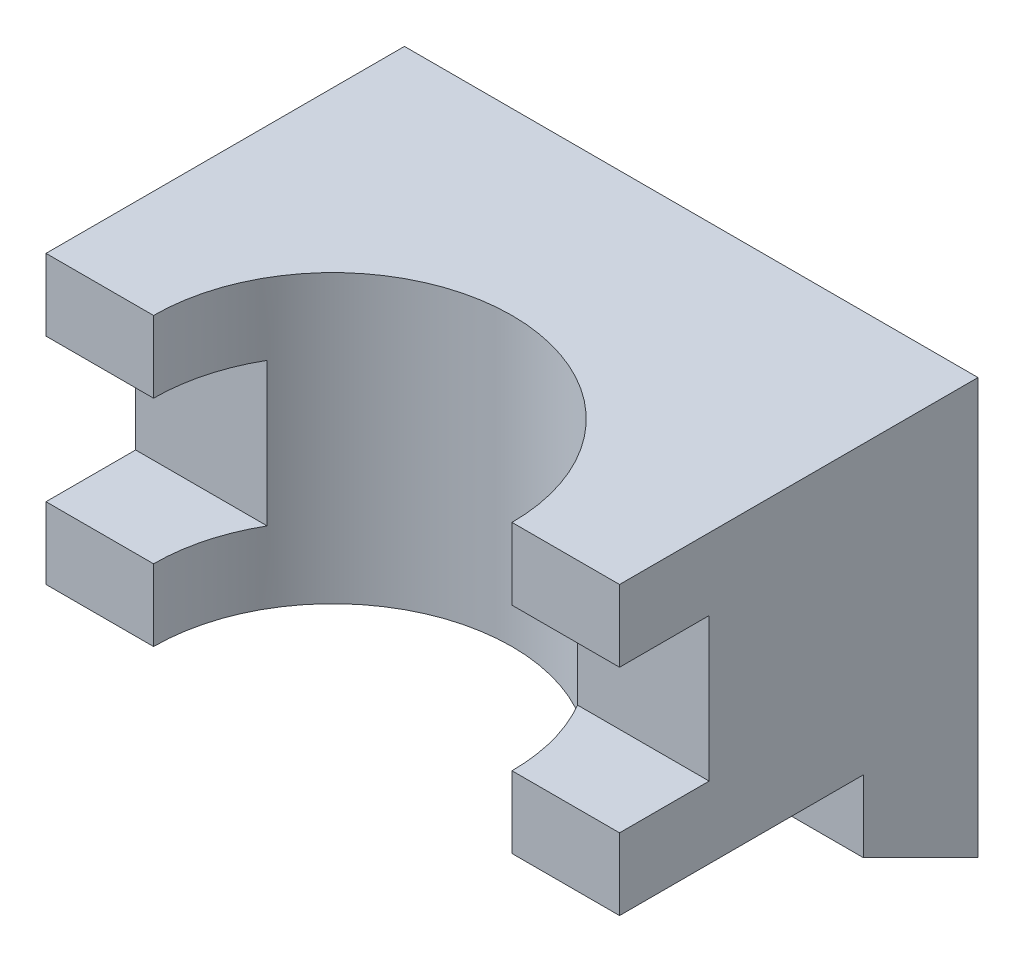
ISO-10303-21;
HEADER;
FILE_DESCRIPTION(('STEP AP214'),'2;1');
FILE_NAME('part.step','',(''),(''),'','','');
FILE_SCHEMA(('AUTOMOTIVE_DESIGN { 1 0 10303 214 1 1 1 1 }'));
ENDSEC;
DATA;
#1=APPLICATION_CONTEXT('core data for automotive mechanical design processes');
#2=APPLICATION_PROTOCOL_DEFINITION('international standard','automotive_design',2000,#1);
#3=PRODUCT_CONTEXT('',#1,'mechanical');
#4=PRODUCT('Part','Part','',(#3));
#5=PRODUCT_RELATED_PRODUCT_CATEGORY('part','',(#4));
#6=PRODUCT_DEFINITION_FORMATION('','',#4);
#7=PRODUCT_DEFINITION_CONTEXT('part definition',#1,'design');
#8=PRODUCT_DEFINITION('design','',#6,#7);
#9=PRODUCT_DEFINITION_SHAPE('','',#8);
#10=(LENGTH_UNIT() NAMED_UNIT(*) SI_UNIT(.MILLI.,.METRE.));
#11=(NAMED_UNIT(*) PLANE_ANGLE_UNIT() SI_UNIT($,.RADIAN.));
#12=(NAMED_UNIT(*) SI_UNIT($,.STERADIAN.) SOLID_ANGLE_UNIT());
#13=UNCERTAINTY_MEASURE_WITH_UNIT(LENGTH_MEASURE(1.E-05),#10,'distance_accuracy_value','');
#14=(GEOMETRIC_REPRESENTATION_CONTEXT(3) GLOBAL_UNCERTAINTY_ASSIGNED_CONTEXT((#13)) GLOBAL_UNIT_ASSIGNED_CONTEXT((#10,
#11,#12)) REPRESENTATION_CONTEXT('',''));
#15=CARTESIAN_POINT('',(0.,0.,0.));
#16=DIRECTION('',(0.,0.,1.));
#17=DIRECTION('',(1.,0.,0.));
#18=AXIS2_PLACEMENT_3D('',#15,#16,#17);
#19=CARTESIAN_POINT('',(80.,-30.,37.5));
#20=DIRECTION('',(0.,1.,0.));
#21=DIRECTION('',(0.,0.,1.));
#22=AXIS2_PLACEMENT_3D('',#19,#20,#21);
#23=PLANE('',#22);
#24=CARTESIAN_POINT('',(40.,-30.,50.));
#25=DIRECTION('',(0.,1.,0.));
#26=DIRECTION('',(0.,0.,1.));
#27=AXIS2_PLACEMENT_3D('',#24,#25,#26);
#28=CIRCLE('',#27,25.);
#29=CARTESIAN_POINT('',(18.349364905389,-30.,37.5));
#30=VERTEX_POINT('',#29);
#31=CARTESIAN_POINT('',(15.,-30.,50.));
#32=VERTEX_POINT('',#31);
#33=EDGE_CURVE('E232',#30,#32,#28,.T.);
#34=ORIENTED_EDGE('',*,*,#33,.F.);
#35=DIRECTION('',(-1.,0.,0.));
#36=VECTOR('',#35,1.);
#37=CARTESIAN_POINT('',(80.,-30.,37.5));
#38=LINE('',#37,#36);
#39=CARTESIAN_POINT('',(0.,-30.,37.5));
#40=VERTEX_POINT('',#39);
#41=EDGE_CURVE('E280',#30,#40,#38,.T.);
#42=ORIENTED_EDGE('',*,*,#41,.T.);
#43=DIRECTION('',(0.,0.,-1.));
#44=VECTOR('',#43,1.);
#45=CARTESIAN_POINT('',(0.,-30.,37.5));
#46=LINE('',#45,#44);
#47=CARTESIAN_POINT('',(0.,-30.,50.));
#48=VERTEX_POINT('',#47);
#49=EDGE_CURVE('E270',#48,#40,#46,.T.);
#50=ORIENTED_EDGE('',*,*,#49,.F.);
#51=DIRECTION('',(-1.,0.,0.));
#52=VECTOR('',#51,1.);
#53=CARTESIAN_POINT('',(80.,-30.,50.));
#54=LINE('',#53,#52);
#55=EDGE_CURVE('E283',#32,#48,#54,.T.);
#56=ORIENTED_EDGE('',*,*,#55,.F.);
#57=EDGE_LOOP('',(#34,#42,#50,#56));
#58=FACE_BOUND('',#57,.T.);
#59=ADVANCED_FACE('F44',(#58),#23,.T.);
#60=CARTESIAN_POINT('',(80.,-30.,50.));
#61=DIRECTION('',(0.,0.,1.));
#62=DIRECTION('',(1.,0.,0.));
#63=AXIS2_PLACEMENT_3D('',#60,#61,#62);
#64=PLANE('',#63);
#65=DIRECTION('',(0.,1.,0.));
#66=VECTOR('',#65,1.);
#67=CARTESIAN_POINT('',(15.,-40.,50.));
#68=LINE('',#67,#66);
#69=CARTESIAN_POINT('',(15.,-40.,50.));
#70=VERTEX_POINT('',#69);
#71=EDGE_CURVE('E240',#70,#32,#68,.T.);
#72=ORIENTED_EDGE('',*,*,#71,.T.);
#73=ORIENTED_EDGE('',*,*,#55,.T.);
#74=DIRECTION('',(0.,1.,0.));
#75=VECTOR('',#74,1.);
#76=CARTESIAN_POINT('',(0.,-30.,50.));
#77=LINE('',#76,#75);
#78=CARTESIAN_POINT('',(0.,-40.,50.));
#79=VERTEX_POINT('',#78);
#80=EDGE_CURVE('E264',#79,#48,#77,.T.);
#81=ORIENTED_EDGE('',*,*,#80,.F.);
#82=DIRECTION('',(-1.,0.,0.));
#83=VECTOR('',#82,1.);
#84=CARTESIAN_POINT('',(80.,-40.,50.));
#85=LINE('',#84,#83);
#86=EDGE_CURVE('E282',#70,#79,#85,.T.);
#87=ORIENTED_EDGE('',*,*,#86,.F.);
#88=EDGE_LOOP('',(#72,#73,#81,#87));
#89=FACE_BOUND('',#88,.T.);
#90=ADVANCED_FACE('F378',(#89),#64,.T.);
#91=CARTESIAN_POINT('',(80.,-10.,37.5));
#92=DIRECTION('',(0.,0.,1.));
#93=DIRECTION('',(1.,0.,0.));
#94=AXIS2_PLACEMENT_3D('',#91,#92,#93);
#95=PLANE('',#94);
#96=DIRECTION('',(0.,1.,0.));
#97=VECTOR('',#96,1.);
#98=CARTESIAN_POINT('',(61.650635094611,-40.,37.5));
#99=LINE('',#98,#97);
#100=CARTESIAN_POINT('',(61.650635094611,-30.,37.5));
#101=VERTEX_POINT('',#100);
#102=CARTESIAN_POINT('',(61.650635094611,-10.,37.5));
#103=VERTEX_POINT('',#102);
#104=EDGE_CURVE('E246',#101,#103,#99,.T.);
#105=ORIENTED_EDGE('',*,*,#104,.F.);
#106=CARTESIAN_POINT('',(80.,-30.,37.5));
#107=VERTEX_POINT('',#106);
#108=EDGE_CURVE('E274',#107,#101,#38,.T.);
#109=ORIENTED_EDGE('',*,*,#108,.F.);
#110=DIRECTION('',(0.,1.,0.));
#111=VECTOR('',#110,1.);
#112=CARTESIAN_POINT('',(80.,-10.,37.5));
#113=LINE('',#112,#111);
#114=CARTESIAN_POINT('',(80.,-10.,37.5));
#115=VERTEX_POINT('',#114);
#116=EDGE_CURVE('E256',#107,#115,#113,.T.);
#117=ORIENTED_EDGE('',*,*,#116,.T.);
#118=DIRECTION('',(-1.,0.,0.));
#119=VECTOR('',#118,1.);
#120=CARTESIAN_POINT('',(80.,-10.,37.5));
#121=LINE('',#120,#119);
#122=EDGE_CURVE('E268',#115,#103,#121,.T.);
#123=ORIENTED_EDGE('',*,*,#122,.T.);
#124=EDGE_LOOP('',(#105,#109,#117,#123));
#125=FACE_BOUND('',#124,.T.);
#126=ADVANCED_FACE('F415',(#125),#95,.T.);
#127=CARTESIAN_POINT('',(40.,-10.,50.));
#128=DIRECTION('',(0.,1.,0.));
#129=DIRECTION('',(0.,0.,1.));
#130=AXIS2_PLACEMENT_3D('',#127,#128,#129);
#131=PLANE('',#130);
#132=DIRECTION('',(0.,0.,1.));
#133=VECTOR('',#132,1.);
#134=CARTESIAN_POINT('',(0.,-10.,16.));
#135=LINE('',#134,#133);
#136=CARTESIAN_POINT('',(0.,-10.,37.5));
#137=VERTEX_POINT('',#136);
#138=CARTESIAN_POINT('',(0.,-10.,50.));
#139=VERTEX_POINT('',#138);
#140=EDGE_CURVE('E305',#137,#139,#135,.T.);
#141=ORIENTED_EDGE('',*,*,#140,.F.);
#142=DIRECTION('',(1.,0.,0.));
#143=VECTOR('',#142,1.);
#144=CARTESIAN_POINT('',(40.,-10.,37.5));
#145=LINE('',#144,#143);
#146=CARTESIAN_POINT('',(18.349364905389,-10.,37.5));
#147=VERTEX_POINT('',#146);
#148=EDGE_CURVE('E345',#137,#147,#145,.T.);
#149=ORIENTED_EDGE('',*,*,#148,.T.);
#150=CARTESIAN_POINT('',(40.,-10.,50.));
#151=DIRECTION('',(0.,-1.,0.));
#152=DIRECTION('',(0.,0.,1.));
#153=AXIS2_PLACEMENT_3D('',#150,#151,#152);
#154=CIRCLE('',#153,25.);
#155=CARTESIAN_POINT('',(15.,-10.,50.));
#156=VERTEX_POINT('',#155);
#157=EDGE_CURVE('E291',#156,#147,#154,.T.);
#158=ORIENTED_EDGE('',*,*,#157,.F.);
#159=DIRECTION('',(1.,0.,0.));
#160=VECTOR('',#159,1.);
#161=CARTESIAN_POINT('',(0.,-10.,50.));
#162=LINE('',#161,#160);
#163=EDGE_CURVE('E289',#139,#156,#162,.T.);
#164=ORIENTED_EDGE('',*,*,#163,.F.);
#165=EDGE_LOOP('',(#141,#149,#158,#164));
#166=FACE_BOUND('',#165,.T.);
#167=ADVANCED_FACE('F393',(#166),#131,.F.);
#168=CARTESIAN_POINT('',(0.,0.,16.));
#169=DIRECTION('',(0.,-1.,0.));
#170=DIRECTION('',(0.,0.,-1.));
#171=AXIS2_PLACEMENT_3D('',#168,#169,#170);
#172=PLANE('',#171);
#173=DIRECTION('',(-1.,0.,0.));
#174=VECTOR('',#173,1.);
#175=CARTESIAN_POINT('',(0.,0.,0.));
#176=LINE('',#175,#174);
#177=CARTESIAN_POINT('',(80.,0.,0.));
#178=VERTEX_POINT('',#177);
#179=CARTESIAN_POINT('',(0.,0.,0.));
#180=VERTEX_POINT('',#179);
#181=EDGE_CURVE('E314',#178,#180,#176,.T.);
#182=ORIENTED_EDGE('',*,*,#181,.T.);
#183=DIRECTION('',(0.,0.,-1.));
#184=VECTOR('',#183,1.);
#185=CARTESIAN_POINT('',(0.,0.,16.));
#186=LINE('',#185,#184);
#187=CARTESIAN_POINT('',(0.,0.,50.));
#188=VERTEX_POINT('',#187);
#189=EDGE_CURVE('E339',#188,#180,#186,.T.);
#190=ORIENTED_EDGE('',*,*,#189,.F.);
#191=DIRECTION('',(1.,0.,0.));
#192=VECTOR('',#191,1.);
#193=CARTESIAN_POINT('',(0.,0.,50.));
#194=LINE('',#193,#192);
#195=CARTESIAN_POINT('',(15.,0.,50.));
#196=VERTEX_POINT('',#195);
#197=EDGE_CURVE('E271',#188,#196,#194,.T.);
#198=ORIENTED_EDGE('',*,*,#197,.T.);
#199=CARTESIAN_POINT('',(40.,0.,50.));
#200=DIRECTION('',(0.,-1.,0.));
#201=DIRECTION('',(0.,0.,1.));
#202=AXIS2_PLACEMENT_3D('',#199,#200,#201);
#203=CIRCLE('',#202,25.);
#204=CARTESIAN_POINT('',(65.,0.,50.));
#205=VERTEX_POINT('',#204);
#206=EDGE_CURVE('E310',#196,#205,#203,.T.);
#207=ORIENTED_EDGE('',*,*,#206,.T.);
#208=DIRECTION('',(1.,0.,0.));
#209=VECTOR('',#208,1.);
#210=CARTESIAN_POINT('',(65.,0.,50.));
#211=LINE('',#210,#209);
#212=CARTESIAN_POINT('',(80.,0.,50.));
#213=VERTEX_POINT('',#212);
#214=EDGE_CURVE('E292',#205,#213,#211,.T.);
#215=ORIENTED_EDGE('',*,*,#214,.T.);
#216=DIRECTION('',(0.,0.,-1.));
#217=VECTOR('',#216,1.);
#218=CARTESIAN_POINT('',(80.,0.,16.));
#219=LINE('',#218,#217);
#220=EDGE_CURVE('E326',#213,#178,#219,.T.);
#221=ORIENTED_EDGE('',*,*,#220,.T.);
#222=EDGE_LOOP('',(#182,#190,#198,#207,#215,#221));
#223=FACE_BOUND('',#222,.T.);
#224=ADVANCED_FACE('F50',(#223),#172,.F.);
#225=CARTESIAN_POINT('',(0.,0.,16.));
#226=DIRECTION('',(1.,0.,0.));
#227=DIRECTION('',(0.,0.,-1.));
#228=AXIS2_PLACEMENT_3D('',#225,#226,#227);
#229=PLANE('',#228);
#230=DIRECTION('',(0.,-1.,0.));
#231=VECTOR('',#230,1.);
#232=CARTESIAN_POINT('',(0.,0.,0.));
#233=LINE('',#232,#231);
#234=CARTESIAN_POINT('',(0.,-58.,0.));
#235=VERTEX_POINT('',#234);
#236=EDGE_CURVE('E332',#180,#235,#233,.T.);
#237=ORIENTED_EDGE('',*,*,#236,.T.);
#238=DIRECTION('',(0.,-0.447213595499958,-0.894427190999916));
#239=VECTOR('',#238,1.);
#240=CARTESIAN_POINT('',(0.,-50.,16.));
#241=LINE('',#240,#239);
#242=CARTESIAN_POINT('',(0.,-50.,16.));
#243=VERTEX_POINT('',#242);
#244=EDGE_CURVE('E222',#243,#235,#241,.T.);
#245=ORIENTED_EDGE('',*,*,#244,.F.);
#246=DIRECTION('',(0.,-1.,0.));
#247=VECTOR('',#246,1.);
#248=CARTESIAN_POINT('',(0.,0.,16.));
#249=LINE('',#248,#247);
#250=CARTESIAN_POINT('',(0.,-40.,16.));
#251=VERTEX_POINT('',#250);
#252=EDGE_CURVE('E325',#251,#243,#249,.T.);
#253=ORIENTED_EDGE('',*,*,#252,.F.);
#254=DIRECTION('',(0.,0.,1.));
#255=VECTOR('',#254,1.);
#256=CARTESIAN_POINT('',(0.,-40.,50.));
#257=LINE('',#256,#255);
#258=EDGE_CURVE('E247',#251,#79,#257,.T.);
#259=ORIENTED_EDGE('',*,*,#258,.T.);
#260=ORIENTED_EDGE('',*,*,#80,.T.);
#261=ORIENTED_EDGE('',*,*,#49,.T.);
#262=DIRECTION('',(0.,1.,0.));
#263=VECTOR('',#262,1.);
#264=CARTESIAN_POINT('',(0.,-10.,37.5));
#265=LINE('',#264,#263);
#266=EDGE_CURVE('E66',#40,#137,#265,.T.);
#267=ORIENTED_EDGE('',*,*,#266,.T.);
#268=ORIENTED_EDGE('',*,*,#140,.T.);
#269=DIRECTION('',(0.,1.,0.));
#270=VECTOR('',#269,1.);
#271=CARTESIAN_POINT('',(0.,-10.,50.));
#272=LINE('',#271,#270);
#273=EDGE_CURVE('E315',#139,#188,#272,.T.);
#274=ORIENTED_EDGE('',*,*,#273,.T.);
#275=ORIENTED_EDGE('',*,*,#189,.T.);
#276=EDGE_LOOP('',(#237,#245,#253,#259,#260,#261,#267,#268,#274,#275));
#277=FACE_BOUND('',#276,.T.);
#278=ADVANCED_FACE('F359',(#277),#229,.F.);
#279=CARTESIAN_POINT('',(80.,0.,16.));
#280=DIRECTION('',(-1.,0.,0.));
#281=DIRECTION('',(0.,0.,1.));
#282=AXIS2_PLACEMENT_3D('',#279,#280,#281);
#283=PLANE('',#282);
#284=DIRECTION('',(0.,1.,0.));
#285=VECTOR('',#284,1.);
#286=CARTESIAN_POINT('',(80.,0.,16.));
#287=LINE('',#286,#285);
#288=CARTESIAN_POINT('',(80.,-50.,16.));
#289=VERTEX_POINT('',#288);
#290=CARTESIAN_POINT('',(80.,-40.,16.));
#291=VERTEX_POINT('',#290);
#292=EDGE_CURVE('E323',#289,#291,#287,.T.);
#293=ORIENTED_EDGE('',*,*,#292,.F.);
#294=DIRECTION('',(0.,-0.447213595499958,-0.894427190999916));
#295=VECTOR('',#294,1.);
#296=CARTESIAN_POINT('',(80.,-50.,16.));
#297=LINE('',#296,#295);
#298=CARTESIAN_POINT('',(80.,-58.,0.));
#299=VERTEX_POINT('',#298);
#300=EDGE_CURVE('E228',#289,#299,#297,.T.);
#301=ORIENTED_EDGE('',*,*,#300,.T.);
#302=DIRECTION('',(0.,1.,0.));
#303=VECTOR('',#302,1.);
#304=CARTESIAN_POINT('',(80.,0.,0.));
#305=LINE('',#304,#303);
#306=EDGE_CURVE('E328',#299,#178,#305,.T.);
#307=ORIENTED_EDGE('',*,*,#306,.T.);
#308=ORIENTED_EDGE('',*,*,#220,.F.);
#309=DIRECTION('',(0.,1.,0.));
#310=VECTOR('',#309,1.);
#311=CARTESIAN_POINT('',(80.,-10.,50.));
#312=LINE('',#311,#310);
#313=CARTESIAN_POINT('',(80.,-10.,50.));
#314=VERTEX_POINT('',#313);
#315=EDGE_CURVE('E317',#314,#213,#312,.T.);
#316=ORIENTED_EDGE('',*,*,#315,.F.);
#317=DIRECTION('',(0.,0.,-1.));
#318=VECTOR('',#317,1.);
#319=CARTESIAN_POINT('',(80.,-10.,50.));
#320=LINE('',#319,#318);
#321=EDGE_CURVE('E299',#314,#115,#320,.T.);
#322=ORIENTED_EDGE('',*,*,#321,.T.);
#323=ORIENTED_EDGE('',*,*,#116,.F.);
#324=DIRECTION('',(0.,0.,-1.));
#325=VECTOR('',#324,1.);
#326=CARTESIAN_POINT('',(80.,-30.,37.5));
#327=LINE('',#326,#325);
#328=CARTESIAN_POINT('',(80.,-30.,50.));
#329=VERTEX_POINT('',#328);
#330=EDGE_CURVE('E257',#329,#107,#327,.T.);
#331=ORIENTED_EDGE('',*,*,#330,.F.);
#332=DIRECTION('',(0.,1.,0.));
#333=VECTOR('',#332,1.);
#334=CARTESIAN_POINT('',(80.,-30.,50.));
#335=LINE('',#334,#333);
#336=CARTESIAN_POINT('',(80.,-40.,50.));
#337=VERTEX_POINT('',#336);
#338=EDGE_CURVE('E254',#337,#329,#335,.T.);
#339=ORIENTED_EDGE('',*,*,#338,.F.);
#340=DIRECTION('',(0.,0.,1.));
#341=VECTOR('',#340,1.);
#342=CARTESIAN_POINT('',(80.,-40.,50.));
#343=LINE('',#342,#341);
#344=EDGE_CURVE('E249',#291,#337,#343,.T.);
#345=ORIENTED_EDGE('',*,*,#344,.F.);
#346=EDGE_LOOP('',(#293,#301,#307,#308,#316,#322,#323,#331,#339,#345));
#347=FACE_BOUND('',#346,.T.);
#348=ADVANCED_FACE('F367',(#347),#283,.F.);
#349=CARTESIAN_POINT('',(0.,0.,16.));
#350=DIRECTION('',(0.,0.,-1.));
#351=DIRECTION('',(-1.,0.,0.));
#352=AXIS2_PLACEMENT_3D('',#349,#350,#351);
#353=PLANE('',#352);
#354=DIRECTION('',(-1.,0.,0.));
#355=VECTOR('',#354,1.);
#356=CARTESIAN_POINT('',(80.,-50.,16.));
#357=LINE('',#356,#355);
#358=CARTESIAN_POINT('',(20.,-50.,16.));
#359=VERTEX_POINT('',#358);
#360=EDGE_CURVE('E230',#359,#243,#357,.T.);
#361=ORIENTED_EDGE('',*,*,#360,.F.);
#362=DIRECTION('',(0.,-1.,0.));
#363=VECTOR('',#362,1.);
#364=CARTESIAN_POINT('',(20.,-45.,16.));
#365=LINE('',#364,#363);
#366=CARTESIAN_POINT('',(20.,-45.,16.));
#367=VERTEX_POINT('',#366);
#368=EDGE_CURVE('E200',#367,#359,#365,.T.);
#369=ORIENTED_EDGE('',*,*,#368,.F.);
#370=DIRECTION('',(-1.,0.,0.));
#371=VECTOR('',#370,1.);
#372=CARTESIAN_POINT('',(60.,-45.,16.));
#373=LINE('',#372,#371);
#374=CARTESIAN_POINT('',(60.,-45.,16.));
#375=VERTEX_POINT('',#374);
#376=EDGE_CURVE('E220',#375,#367,#373,.T.);
#377=ORIENTED_EDGE('',*,*,#376,.F.);
#378=DIRECTION('',(0.,1.,0.));
#379=VECTOR('',#378,1.);
#380=CARTESIAN_POINT('',(60.,-50.,16.));
#381=LINE('',#380,#379);
#382=CARTESIAN_POINT('',(60.,-50.,16.));
#383=VERTEX_POINT('',#382);
#384=EDGE_CURVE('E204',#383,#375,#381,.T.);
#385=ORIENTED_EDGE('',*,*,#384,.F.);
#386=EDGE_CURVE('E233',#289,#383,#357,.T.);
#387=ORIENTED_EDGE('',*,*,#386,.F.);
#388=ORIENTED_EDGE('',*,*,#292,.T.);
#389=DIRECTION('',(-1.,0.,0.));
#390=VECTOR('',#389,1.);
#391=CARTESIAN_POINT('',(80.,-40.,16.));
#392=LINE('',#391,#390);
#393=EDGE_CURVE('E263',#291,#251,#392,.T.);
#394=ORIENTED_EDGE('',*,*,#393,.T.);
#395=ORIENTED_EDGE('',*,*,#252,.T.);
#396=EDGE_LOOP('',(#361,#369,#377,#385,#387,#388,#394,#395));
#397=FACE_BOUND('',#396,.T.);
#398=ADVANCED_FACE('F357',(#397),#353,.F.);
#399=CARTESIAN_POINT('',(0.,0.,0.));
#400=DIRECTION('',(0.,0.,-1.));
#401=DIRECTION('',(-1.,0.,0.));
#402=AXIS2_PLACEMENT_3D('',#399,#400,#401);
#403=PLANE('',#402);
#404=ORIENTED_EDGE('',*,*,#181,.F.);
#405=ORIENTED_EDGE('',*,*,#306,.F.);
#406=DIRECTION('',(1.,0.,0.));
#407=VECTOR('',#406,1.);
#408=CARTESIAN_POINT('',(80.,-58.,0.));
#409=LINE('',#408,#407);
#410=EDGE_CURVE('E331',#235,#299,#409,.T.);
#411=ORIENTED_EDGE('',*,*,#410,.F.);
#412=ORIENTED_EDGE('',*,*,#236,.F.);
#413=EDGE_LOOP('',(#404,#405,#411,#412));
#414=FACE_BOUND('',#413,.T.);
#415=ADVANCED_FACE('F362',(#414),#403,.T.);
#416=CARTESIAN_POINT('',(0.,-10.,50.));
#417=DIRECTION('',(0.,0.,1.));
#418=DIRECTION('',(1.,0.,0.));
#419=AXIS2_PLACEMENT_3D('',#416,#417,#418);
#420=PLANE('',#419);
#421=ORIENTED_EDGE('',*,*,#197,.F.);
#422=ORIENTED_EDGE('',*,*,#273,.F.);
#423=ORIENTED_EDGE('',*,*,#163,.T.);
#424=DIRECTION('',(0.,1.,0.));
#425=VECTOR('',#424,1.);
#426=CARTESIAN_POINT('',(15.,-10.,50.));
#427=LINE('',#426,#425);
#428=EDGE_CURVE('E302',#156,#196,#427,.T.);
#429=ORIENTED_EDGE('',*,*,#428,.T.);
#430=EDGE_LOOP('',(#421,#422,#423,#429));
#431=FACE_BOUND('',#430,.T.);
#432=ADVANCED_FACE('F392',(#431),#420,.T.);
#433=CARTESIAN_POINT('',(65.,-10.,50.));
#434=DIRECTION('',(0.,0.,1.));
#435=DIRECTION('',(1.,0.,0.));
#436=AXIS2_PLACEMENT_3D('',#433,#434,#435);
#437=PLANE('',#436);
#438=ORIENTED_EDGE('',*,*,#214,.F.);
#439=DIRECTION('',(0.,1.,0.));
#440=VECTOR('',#439,1.);
#441=CARTESIAN_POINT('',(65.,-10.,50.));
#442=LINE('',#441,#440);
#443=CARTESIAN_POINT('',(65.,-10.,50.));
#444=VERTEX_POINT('',#443);
#445=EDGE_CURVE('E316',#444,#205,#442,.T.);
#446=ORIENTED_EDGE('',*,*,#445,.F.);
#447=DIRECTION('',(1.,0.,0.));
#448=VECTOR('',#447,1.);
#449=CARTESIAN_POINT('',(65.,-10.,50.));
#450=LINE('',#449,#448);
#451=EDGE_CURVE('E298',#444,#314,#450,.T.);
#452=ORIENTED_EDGE('',*,*,#451,.T.);
#453=ORIENTED_EDGE('',*,*,#315,.T.);
#454=EDGE_LOOP('',(#438,#446,#452,#453));
#455=FACE_BOUND('',#454,.T.);
#456=ADVANCED_FACE('F402',(#455),#437,.T.);
#457=CARTESIAN_POINT('',(40.,-10.,50.));
#458=DIRECTION('',(0.,1.,0.));
#459=DIRECTION('',(0.,0.,1.));
#460=AXIS2_PLACEMENT_3D('',#457,#458,#459);
#461=CYLINDRICAL_SURFACE('',#460,25.);
#462=ORIENTED_EDGE('',*,*,#206,.F.);
#463=ORIENTED_EDGE('',*,*,#428,.F.);
#464=ORIENTED_EDGE('',*,*,#157,.T.);
#465=DIRECTION('',(0.,1.,0.));
#466=VECTOR('',#465,1.);
#467=CARTESIAN_POINT('',(18.349364905389,-40.,37.5));
#468=LINE('',#467,#466);
#469=EDGE_CURVE('E244',#30,#147,#468,.T.);
#470=ORIENTED_EDGE('',*,*,#469,.F.);
#471=ORIENTED_EDGE('',*,*,#33,.T.);
#472=ORIENTED_EDGE('',*,*,#71,.F.);
#473=CARTESIAN_POINT('',(40.,-40.,50.));
#474=DIRECTION('',(0.,1.,0.));
#475=DIRECTION('',(0.,0.,1.));
#476=AXIS2_PLACEMENT_3D('',#473,#474,#475);
#477=CIRCLE('',#476,25.);
#478=CARTESIAN_POINT('',(65.,-40.,50.));
#479=VERTEX_POINT('',#478);
#480=EDGE_CURVE('E241',#479,#70,#477,.T.);
#481=ORIENTED_EDGE('',*,*,#480,.F.);
#482=DIRECTION('',(0.,1.,0.));
#483=VECTOR('',#482,1.);
#484=CARTESIAN_POINT('',(65.,-40.,50.));
#485=LINE('',#484,#483);
#486=CARTESIAN_POINT('',(65.,-30.,50.));
#487=VERTEX_POINT('',#486);
#488=EDGE_CURVE('E238',#479,#487,#485,.T.);
#489=ORIENTED_EDGE('',*,*,#488,.T.);
#490=CARTESIAN_POINT('',(40.,-30.,50.));
#491=DIRECTION('',(0.,1.,0.));
#492=DIRECTION('',(0.,0.,1.));
#493=AXIS2_PLACEMENT_3D('',#490,#491,#492);
#494=CIRCLE('',#493,25.);
#495=EDGE_CURVE('E234',#487,#101,#494,.T.);
#496=ORIENTED_EDGE('',*,*,#495,.T.);
#497=ORIENTED_EDGE('',*,*,#104,.T.);
#498=EDGE_CURVE('E293',#103,#444,#154,.T.);
#499=ORIENTED_EDGE('',*,*,#498,.T.);
#500=ORIENTED_EDGE('',*,*,#445,.T.);
#501=EDGE_LOOP('',(#462,#463,#464,#470,#471,#472,#481,#489,#496,#497,#499,#500));
#502=FACE_BOUND('',#501,.T.);
#503=ADVANCED_FACE('F418',(#502),#461,.F.);
#504=ORIENTED_EDGE('',*,*,#498,.F.);
#505=ORIENTED_EDGE('',*,*,#122,.F.);
#506=ORIENTED_EDGE('',*,*,#321,.F.);
#507=ORIENTED_EDGE('',*,*,#451,.F.);
#508=EDGE_LOOP('',(#504,#505,#506,#507));
#509=FACE_BOUND('',#508,.T.);
#510=ADVANCED_FACE('F407',(#509),#131,.F.);
#511=ORIENTED_EDGE('',*,*,#469,.T.);
#512=ORIENTED_EDGE('',*,*,#148,.F.);
#513=ORIENTED_EDGE('',*,*,#266,.F.);
#514=ORIENTED_EDGE('',*,*,#41,.F.);
#515=EDGE_LOOP('',(#511,#512,#513,#514));
#516=FACE_BOUND('',#515,.T.);
#517=ADVANCED_FACE('F387',(#516),#95,.T.);
#518=ORIENTED_EDGE('',*,*,#495,.F.);
#519=EDGE_CURVE('E279',#329,#487,#54,.T.);
#520=ORIENTED_EDGE('',*,*,#519,.F.);
#521=ORIENTED_EDGE('',*,*,#330,.T.);
#522=ORIENTED_EDGE('',*,*,#108,.T.);
#523=EDGE_LOOP('',(#518,#520,#521,#522));
#524=FACE_BOUND('',#523,.T.);
#525=ADVANCED_FACE('F412',(#524),#23,.T.);
#526=ORIENTED_EDGE('',*,*,#488,.F.);
#527=EDGE_CURVE('E285',#337,#479,#85,.T.);
#528=ORIENTED_EDGE('',*,*,#527,.F.);
#529=ORIENTED_EDGE('',*,*,#338,.T.);
#530=ORIENTED_EDGE('',*,*,#519,.T.);
#531=EDGE_LOOP('',(#526,#528,#529,#530));
#532=FACE_BOUND('',#531,.T.);
#533=ADVANCED_FACE('F419',(#532),#64,.T.);
#534=CARTESIAN_POINT('',(80.,-40.,50.));
#535=DIRECTION('',(0.,-1.,0.));
#536=DIRECTION('',(0.,0.,-1.));
#537=AXIS2_PLACEMENT_3D('',#534,#535,#536);
#538=PLANE('',#537);
#539=ORIENTED_EDGE('',*,*,#480,.T.);
#540=ORIENTED_EDGE('',*,*,#86,.T.);
#541=ORIENTED_EDGE('',*,*,#258,.F.);
#542=ORIENTED_EDGE('',*,*,#393,.F.);
#543=ORIENTED_EDGE('',*,*,#344,.T.);
#544=ORIENTED_EDGE('',*,*,#527,.T.);
#545=EDGE_LOOP('',(#539,#540,#541,#542,#543,#544));
#546=FACE_BOUND('',#545,.T.);
#547=ADVANCED_FACE('F372',(#546),#538,.T.);
#548=CARTESIAN_POINT('',(80.,-50.,16.));
#549=DIRECTION('',(0.,0.894427190999916,-0.447213595499958));
#550=DIRECTION('',(0.,0.447213595499958,0.894427190999916));
#551=AXIS2_PLACEMENT_3D('',#548,#549,#550);
#552=PLANE('',#551);
#553=DIRECTION('',(-1.,0.,0.));
#554=VECTOR('',#553,1.);
#555=CARTESIAN_POINT('',(80.,-55.,5.99999999999998));
#556=LINE('',#555,#554);
#557=CARTESIAN_POINT('',(60.,-55.,5.99999999999998));
#558=VERTEX_POINT('',#557);
#559=CARTESIAN_POINT('',(20.,-55.,5.99999999999996));
#560=VERTEX_POINT('',#559);
#561=EDGE_CURVE('E52',#558,#560,#556,.T.);
#562=ORIENTED_EDGE('',*,*,#561,.T.);
#563=DIRECTION('',(0.,0.447213595499958,0.894427190999916));
#564=VECTOR('',#563,1.);
#565=CARTESIAN_POINT('',(20.,-50.,16.));
#566=LINE('',#565,#564);
#567=EDGE_CURVE('E11',#560,#359,#566,.T.);
#568=ORIENTED_EDGE('',*,*,#567,.T.);
#569=ORIENTED_EDGE('',*,*,#360,.T.);
#570=ORIENTED_EDGE('',*,*,#244,.T.);
#571=ORIENTED_EDGE('',*,*,#410,.T.);
#572=ORIENTED_EDGE('',*,*,#300,.F.);
#573=ORIENTED_EDGE('',*,*,#386,.T.);
#574=DIRECTION('',(0.,-0.447213595499958,-0.894427190999916));
#575=VECTOR('',#574,1.);
#576=CARTESIAN_POINT('',(60.,-50.,16.));
#577=LINE('',#576,#575);
#578=EDGE_CURVE('E343',#383,#558,#577,.T.);
#579=ORIENTED_EDGE('',*,*,#578,.T.);
#580=EDGE_LOOP('',(#562,#568,#569,#570,#571,#572,#573,#579));
#581=FACE_BOUND('',#580,.T.);
#582=ADVANCED_FACE('F349',(#581),#552,.F.);
#583=CARTESIAN_POINT('',(20.,-55.,5.));
#584=DIRECTION('',(0.,-1.,0.));
#585=DIRECTION('',(0.,0.,-1.));
#586=AXIS2_PLACEMENT_3D('',#583,#584,#585);
#587=PLANE('',#586);
#588=DIRECTION('',(0.,0.,1.));
#589=VECTOR('',#588,1.);
#590=CARTESIAN_POINT('',(60.,-55.,5.));
#591=LINE('',#590,#589);
#592=CARTESIAN_POINT('',(60.,-55.,5.));
#593=VERTEX_POINT('',#592);
#594=EDGE_CURVE('E58',#593,#558,#591,.T.);
#595=ORIENTED_EDGE('',*,*,#594,.F.);
#596=DIRECTION('',(1.,0.,0.));
#597=VECTOR('',#596,1.);
#598=CARTESIAN_POINT('',(20.,-55.,5.));
#599=LINE('',#598,#597);
#600=CARTESIAN_POINT('',(20.,-55.,5.));
#601=VERTEX_POINT('',#600);
#602=EDGE_CURVE('E198',#601,#593,#599,.T.);
#603=ORIENTED_EDGE('',*,*,#602,.F.);
#604=DIRECTION('',(0.,0.,1.));
#605=VECTOR('',#604,1.);
#606=CARTESIAN_POINT('',(20.,-55.,5.));
#607=LINE('',#606,#605);
#608=EDGE_CURVE('E225',#601,#560,#607,.T.);
#609=ORIENTED_EDGE('',*,*,#608,.T.);
#610=ORIENTED_EDGE('',*,*,#561,.F.);
#611=EDGE_LOOP('',(#595,#603,#609,#610));
#612=FACE_BOUND('',#611,.T.);
#613=ADVANCED_FACE('F355',(#612),#587,.F.);
#614=CARTESIAN_POINT('',(20.,-45.,5.));
#615=DIRECTION('',(-1.,0.,0.));
#616=DIRECTION('',(0.,0.,1.));
#617=AXIS2_PLACEMENT_3D('',#614,#615,#616);
#618=PLANE('',#617);
#619=ORIENTED_EDGE('',*,*,#608,.F.);
#620=DIRECTION('',(0.,-1.,0.));
#621=VECTOR('',#620,1.);
#622=CARTESIAN_POINT('',(20.,-45.,5.));
#623=LINE('',#622,#621);
#624=CARTESIAN_POINT('',(20.,-45.,5.));
#625=VERTEX_POINT('',#624);
#626=EDGE_CURVE('E212',#625,#601,#623,.T.);
#627=ORIENTED_EDGE('',*,*,#626,.F.);
#628=DIRECTION('',(0.,0.,1.));
#629=VECTOR('',#628,1.);
#630=CARTESIAN_POINT('',(20.,-45.,5.));
#631=LINE('',#630,#629);
#632=EDGE_CURVE('E210',#625,#367,#631,.T.);
#633=ORIENTED_EDGE('',*,*,#632,.T.);
#634=ORIENTED_EDGE('',*,*,#368,.T.);
#635=ORIENTED_EDGE('',*,*,#567,.F.);
#636=EDGE_LOOP('',(#619,#627,#633,#634,#635));
#637=FACE_BOUND('',#636,.T.);
#638=ADVANCED_FACE('F351',(#637),#618,.F.);
#639=CARTESIAN_POINT('',(60.,-50.,5.));
#640=DIRECTION('',(1.,0.,0.));
#641=DIRECTION('',(0.,0.,-1.));
#642=AXIS2_PLACEMENT_3D('',#639,#640,#641);
#643=PLANE('',#642);
#644=ORIENTED_EDGE('',*,*,#384,.T.);
#645=DIRECTION('',(0.,0.,1.));
#646=VECTOR('',#645,1.);
#647=CARTESIAN_POINT('',(60.,-45.,5.));
#648=LINE('',#647,#646);
#649=CARTESIAN_POINT('',(60.,-45.,5.));
#650=VERTEX_POINT('',#649);
#651=EDGE_CURVE('E197',#650,#375,#648,.T.);
#652=ORIENTED_EDGE('',*,*,#651,.F.);
#653=DIRECTION('',(0.,1.,0.));
#654=VECTOR('',#653,1.);
#655=CARTESIAN_POINT('',(60.,-55.,5.));
#656=LINE('',#655,#654);
#657=EDGE_CURVE('E186',#593,#650,#656,.T.);
#658=ORIENTED_EDGE('',*,*,#657,.F.);
#659=ORIENTED_EDGE('',*,*,#594,.T.);
#660=ORIENTED_EDGE('',*,*,#578,.F.);
#661=EDGE_LOOP('',(#644,#652,#658,#659,#660));
#662=FACE_BOUND('',#661,.T.);
#663=ADVANCED_FACE('F202',(#662),#643,.F.);
#664=CARTESIAN_POINT('',(60.,-45.,5.));
#665=DIRECTION('',(0.,1.,0.));
#666=DIRECTION('',(0.,0.,1.));
#667=AXIS2_PLACEMENT_3D('',#664,#665,#666);
#668=PLANE('',#667);
#669=ORIENTED_EDGE('',*,*,#376,.T.);
#670=ORIENTED_EDGE('',*,*,#632,.F.);
#671=DIRECTION('',(-1.,0.,0.));
#672=VECTOR('',#671,1.);
#673=CARTESIAN_POINT('',(60.,-45.,5.));
#674=LINE('',#673,#672);
#675=EDGE_CURVE('E191',#650,#625,#674,.T.);
#676=ORIENTED_EDGE('',*,*,#675,.F.);
#677=ORIENTED_EDGE('',*,*,#651,.T.);
#678=EDGE_LOOP('',(#669,#670,#676,#677));
#679=FACE_BOUND('',#678,.T.);
#680=ADVANCED_FACE('F209',(#679),#668,.F.);
#681=CARTESIAN_POINT('',(0.,0.,5.));
#682=DIRECTION('',(0.,0.,1.));
#683=DIRECTION('',(1.,0.,0.));
#684=AXIS2_PLACEMENT_3D('',#681,#682,#683);
#685=PLANE('',#684);
#686=ORIENTED_EDGE('',*,*,#657,.T.);
#687=ORIENTED_EDGE('',*,*,#675,.T.);
#688=ORIENTED_EDGE('',*,*,#626,.T.);
#689=ORIENTED_EDGE('',*,*,#602,.T.);
#690=EDGE_LOOP('',(#686,#687,#688,#689));
#691=FACE_BOUND('',#690,.T.);
#692=ADVANCED_FACE('F192',(#691),#685,.T.);
#693=CLOSED_SHELL('',(#59,#90,#126,#167,#224,#278,#348,#398,#415,#432,#456,#503,#510,#517,#525,
#533,#547,#582,#613,#638,#663,#680,#692));
#694=MANIFOLD_SOLID_BREP('B2',#693);
#695=ADVANCED_BREP_SHAPE_REPRESENTATION('',(#18,#694),#14);
#696=SHAPE_DEFINITION_REPRESENTATION(#9,#695);
ENDSEC;
END-ISO-10303-21;
